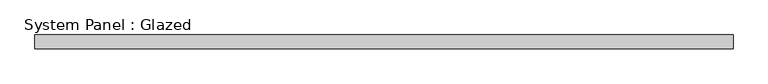
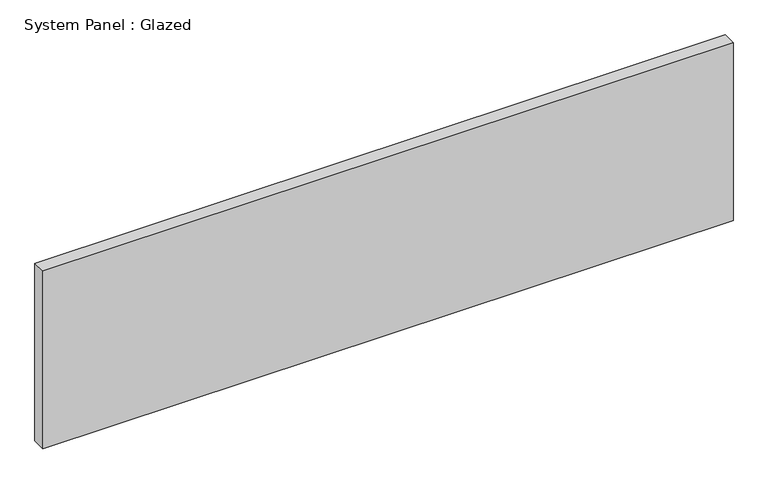
"""IFC4 building model written with IfcOpenShell, lengths in millimetres: plate geometry, System Panel : Glazed."""

from ifc_helpers import new_model, si_unit, origin, origin_with_axes, place, context, project, spatial, polyline, outline, extrude, source, transform, mapped, element, save


def system_panel_glazed_6984195a(model_context):
    return source(origin(), model_context, "Body", "SweptSolid", [
        extrude(outline(polyline([(641.35, 19.05), (-641.35, 19.05), (-641.35, 44.45), (641.35, 44.45), (641.35, 19.05)])), origin_with_axes(), (0.0, 0.0, 1.0), 349.25),
    ])


if __name__ == "__main__":
    model = new_model("IFC4")
    model_context = context("Model", 3, world=origin())
    ifc_project = project(units=[si_unit("LENGTHUNIT", "METRE", prefix="MILLI")], contexts=[model_context])
    site = spatial("IfcSite", under=ifc_project)
    building = spatial("IfcBuilding", under=site)
    placement = place(None, origin())
    system_panel_glazed_shape = system_panel_glazed_6984195a(model_context)
    element("IfcPlate", 1, ObjectType="System Panel : Glazed", at=placement, inside=building, context=model_context, shape_type="MappedRepresentation", body=[
        mapped(system_panel_glazed_shape, transform((0.0, 0.0, 0.0), x_axis=(1.0, 0.0, 0.0), y_axis=(0.0, 1.0, 0.0), z_axis=(0.0, 0.0, 1.0))),
    ])
    save(model, "model.ifc")

# Revit data of these elements
# Type "System Panel : Glazed"
#   Construction Type Id = "GSP4R"
#   Analytic Construction = "1/8 in Pilkington single glazing"
#   Visual Light Transmittance = 0.9
#   Solar Heat Gain Coefficient = 0.86
#   Heat Transfer Coefficient (U) = 1.18115 BTU/(h·ft²·°F)
#   Define Thermal Properties by = 1
# Element 1 (IfcPlate, "System Panel : Glazed")
#   Materials on its faces: "Glass"
# Materials
#   "Glass": class "Glass", colour RGB 0 128 192, transparency 0.75, Description = "Soda Lime Glass", Cost = 0
